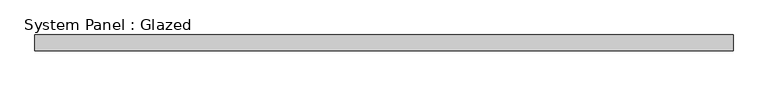
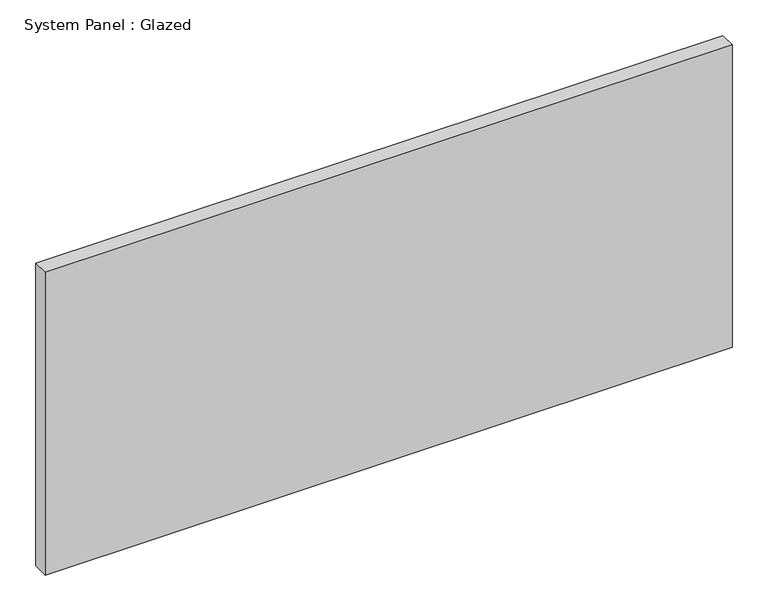
"""IFC4 building model written with IfcOpenShell, lengths in millimetres: plate geometry, System Panel : Glazed."""

from ifc_helpers import new_model, si_unit, origin, origin_with_axes, place, context, project, spatial, polyline, outline, extrude, source, transform, mapped, element, save


def system_panel_glazed_d57d3c71(model_context):
    return source(origin(), model_context, "Body", "SweptSolid", [
        extrude(outline(polyline([(552.4499999, 19.05), (-552.4499999, 19.05), (-552.4499999, 44.45), (552.4499999, 44.45), (552.4499999, 19.05)])), origin_with_axes(), (0.0, 0.0, 1.0), 514.35),
    ])


if __name__ == "__main__":
    model = new_model("IFC4")
    model_context = context("Model", 3, world=origin())
    ifc_project = project(units=[si_unit("LENGTHUNIT", "METRE", prefix="MILLI")], contexts=[model_context])
    site = spatial("IfcSite", under=ifc_project)
    building = spatial("IfcBuilding", under=site)
    placement = place(None, origin())
    system_panel_glazed_shape = system_panel_glazed_d57d3c71(model_context)
    element("IfcPlate", 1, ObjectType="System Panel : Glazed", at=placement, inside=building, context=model_context, shape_type="MappedRepresentation", body=[
        mapped(system_panel_glazed_shape, transform((0.0, 0.0, 0.0), x_axis=(1.0, 0.0, 0.0), y_axis=(0.0, 1.0, 0.0), z_axis=(0.0, 0.0, 1.0))),
    ])
    save(model, "model.ifc")

# Revit data of these elements
# Type "System Panel : Glazed"
#   Construction Type Id = "GSP4R"
#   Analytic Construction = "1/8 in Pilkington single glazing"
#   Visual Light Transmittance = 0.9
#   Solar Heat Gain Coefficient = 0.86
#   Heat Transfer Coefficient (U) = 1.18115 BTU/(h·ft²·°F)
#   Define Thermal Properties by = 1
# Element 1 (IfcPlate, "System Panel : Glazed")
#   Materials on its faces: "glass panel 223"
# Materials
#   "glass panel 223": class "Generic", colour RGB 120 120 120, transparency 0, Cost = 0
